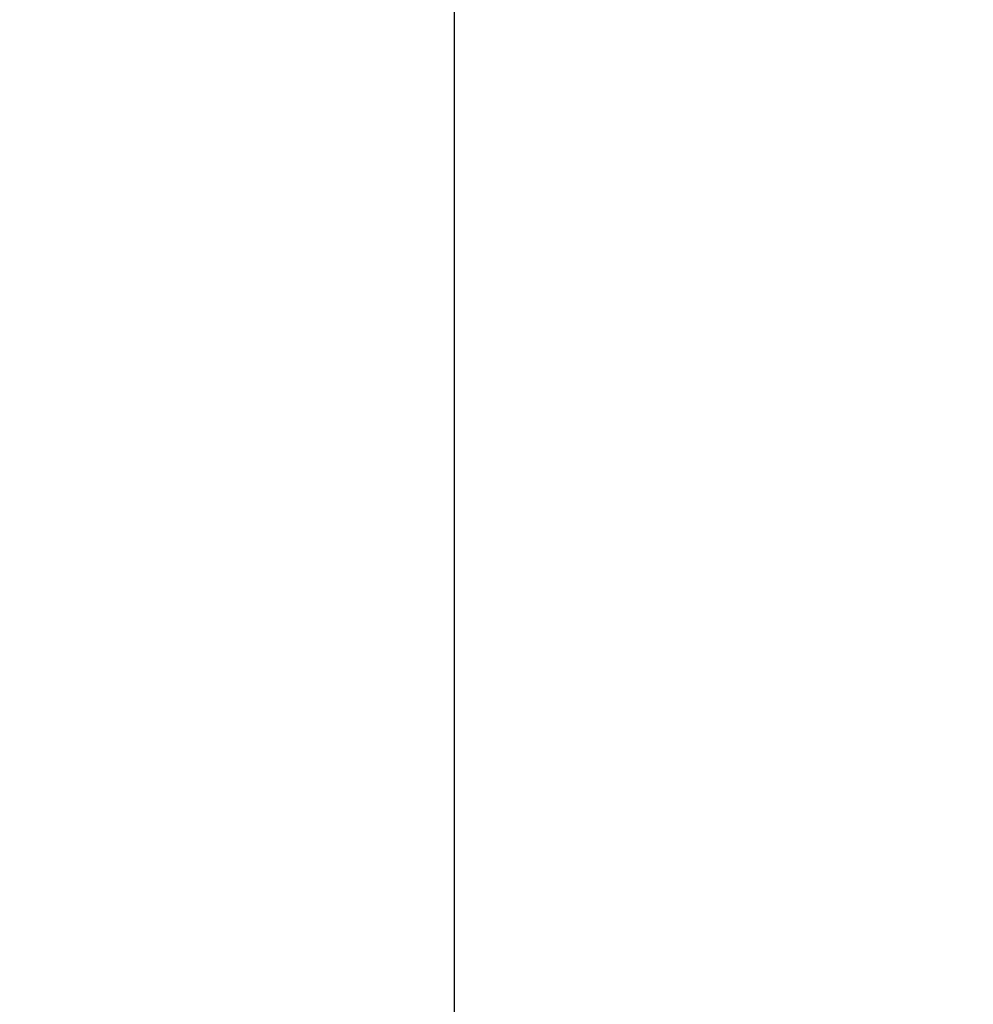
# Model space of a CAD drawing. Units: inches. Extents: x 2083 to 3317, y 1141 to 2115.
# Tile 125 of 256: x 3119.67 to 3135.66, y 1238.34 to 1254.86. Entities that reach past the tile are written whole.
import ezdxf

# ---------------------------------------------------------------- set-up
doc = ezdxf.new("R2010")
doc.units = ezdxf.units.IN
doc.layers.add('A-ANNO-DIMS', color=2, linetype='Continuous', lineweight=18)
doc.styles.get("Standard").update_dxf_attribs({"font": 'arial.ttf'})
doc.dimstyles.new('ISO-25', dxfattribs={"dimtxt": 12, "dimasz": 12, "dimexe": 1.25, "dimexo": 0.625, "dimtad": 1, "dimlunit": 3, "dimtxsty": 'Standard', "dimcen": 2.5, "dimadec": 0, "dimazin": 0, "dimtfac": 1, "dimtmove": 0, "dimatfit": 3, "dimfxl": 1, "dimarcsym": 0})

# ---------------------------------------------------------------- blocks, each defined once
blk = doc.blocks.new('*D10')
at = {"layer": 'A-ANNO-DIMS', "color": 0, "lineweight": -2, "transparency": 16777216}
for p, q in [((2862.96, 1262.636), (2862.96, 1201.384)), ((3126.96, 1262.636), (3126.96, 1201.384)), ((2874.96, 1202.634), (3114.96, 1202.634))]:
    blk.add_line(p, q, dxfattribs=at)
at = {"layer": 'A-ANNO-DIMS', "color": 0, "transparency": 16777216}
for points in [[(2874.96, 1204.634), (2874.96, 1200.634), (2862.96, 1202.634)], [(3114.96, 1204.634), (3114.96, 1200.634), (3126.96, 1202.634)]]:
    blk.add_solid(points, dxfattribs=at)
at = {"layer": 'Defpoints', "color": 0, "transparency": 16777216}
for p in [(2862.96, 1263.261), (3126.96, 1263.261), (3126.96, 1202.634)]:
    blk.add_point(p, dxfattribs=at)
at = {"layer": 'A-ANNO-DIMS', "color": 0, "transparency": 16777216, "insert": (2994.96, 1209.284), "char_height": 12, "attachment_point": 5}
blk.add_mtext("22'", dxfattribs=at)
blk = doc.blocks.new('*D26')
at = {"layer": 'A-ANNO-DIMS', "color": 0, "lineweight": -2, "transparency": 16777216}
for p, q in [((3088.986, 1274.915), (3088.986, 1270.952)), ((3111.24, 1274.915), (3111.24, 1270.952)), ((3076.986, 1272.202), (2840.262, 1272.202)), ((3111.24, 1272.202), (3088.986, 1272.202)), ((3123.24, 1272.202), (3135.24, 1272.202))]:
    blk.add_line(p, q, dxfattribs=at)
at = {"layer": 'A-ANNO-DIMS', "color": 0, "transparency": 16777216}
for points in [[(3076.986, 1274.202), (3076.986, 1270.202), (3088.986, 1272.202)], [(3123.24, 1274.202), (3123.24, 1270.202), (3111.24, 1272.202)]]:
    blk.add_solid(points, dxfattribs=at)
at = {"layer": 'Defpoints', "color": 0, "transparency": 16777216}
for p in [(3088.986, 1275.54), (3111.24, 1275.54), (3088.986, 1272.202)]:
    blk.add_point(p, dxfattribs=at)
at = {"layer": 'A-ANNO-DIMS', "color": 0, "transparency": 16777216, "insert": (2952.624, 1279.032), "char_height": 12, "attachment_point": 5}
blk.add_mtext('NIGHTSTAND 1\'-10 1/2" TYP.', dxfattribs=at)
blk = doc.blocks.new('*D27')
at = {"layer": 'A-ANNO-DIMS', "color": 0, "lineweight": -2, "transparency": 16777216}
for p, q in [((3114.578, 1309.794), (3114.578, 1321.794)), ((3111.865, 1297.794), (3115.828, 1297.794)), ((3114.578, 1297.794), (3114.578, 1275.54)), ((3111.865, 1275.54), (3115.828, 1275.54)), ((3114.578, 1263.54), (3114.578, 1140.989))]:
    blk.add_line(p, q, dxfattribs=at)
at = {"layer": 'A-ANNO-DIMS', "color": 0, "transparency": 16777216}
for points in [[(3112.578, 1309.794), (3116.578, 1309.794), (3114.578, 1297.794)], [(3112.578, 1263.54), (3116.578, 1263.54), (3114.578, 1275.54)]]:
    blk.add_solid(points, dxfattribs=at)
at = {"layer": 'Defpoints', "color": 0, "transparency": 16777216}
for p in [(3111.24, 1297.794), (3111.24, 1275.54), (3114.578, 1275.54)]:
    blk.add_point(p, dxfattribs=at)
at = {"layer": 'A-ANNO-DIMS', "color": 0, "transparency": 16777216, "insert": (3107.749, 1196.264), "char_height": 12, "attachment_point": 5, "rotation": 90}
blk.add_mtext('1\'-10 1/2" TYP.', dxfattribs=at)
blk = doc.blocks.new('*D34')
at = {"layer": 'A-ANNO-DIMS', "color": 0, "lineweight": -2, "transparency": 16777216}
for p, q in [((2226.96, 1262.636), (2226.96, 1209.661)), ((3126.96, 1262.636), (3126.96, 1209.661)), ((2238.96, 1210.911), (3114.96, 1210.911))]:
    blk.add_line(p, q, dxfattribs=at)
at = {"layer": 'A-ANNO-DIMS', "color": 0, "transparency": 16777216}
for points in [[(2238.96, 1212.911), (2238.96, 1208.911), (2226.96, 1210.911)], [(3114.96, 1212.911), (3114.96, 1208.911), (3126.96, 1210.911)]]:
    blk.add_solid(points, dxfattribs=at)
at = {"layer": 'Defpoints', "color": 0, "transparency": 16777216}
for p in [(2226.96, 1263.261), (3126.96, 1263.261), (3126.96, 1210.911)]:
    blk.add_point(p, dxfattribs=at)
at = {"layer": 'A-ANNO-DIMS', "color": 0, "transparency": 16777216, "insert": (2676.96, 1217.663), "char_height": 12, "attachment_point": 5}
blk.add_mtext('75\'-0"', dxfattribs=at)

msp = doc.modelspace()

# ---------------------------------------------------------------- dimensions: what is measured, and where the dimension line sits
at = {"layer": 'A-ANNO-DIMS'}
for base, p1, p2, angle, text, picture, middle in [((3114.578, 1275.54), (3111.24, 1297.794), (3111.24, 1275.54), 270, '<> TYP.', '*D27', (3107.749, 1196.264)), ((3088.986, 1272.202), (3111.24, 1275.54), (3088.986, 1275.54), 180, 'NIGHTSTAND <> TYP.', '*D26', (2952.624, 1279.032))]:
    dim = msp.add_linear_dim(base=base, p1=p1, p2=p2, angle=angle, text=text, dimstyle='ISO-25', override={"dimdec": 1, "dimlfac": 1, "dimrnd": 0, "dimzin": 1, "dimdsep": 46, "dimlunit": 4, "dimfrac": 2}, dxfattribs=at)
    dim.commit()
    dim.dimension.update_dxf_attribs({"geometry": picture, "text_midpoint": middle})
for base, p1, override, picture, middle in [((3126.96, 1210.911), (2226.96, 1263.261), {"dimdec": 1, "dimlfac": 1, "dimrnd": 0, "dimzin": 1, "dimdsep": 46, "dimlunit": 4, "dimfrac": 2}, '*D34', (2676.96, 1217.663)), ((3126.96, 1202.634), (2862.96, 1263.261), {"dimclrd": 0, "dimclre": 0, "dimclrt": 0}, '*D10', (2994.96, 1209.284))]:
    dim = msp.add_linear_dim(base=base, p1=p1, p2=(3126.96, 1263.261), dimstyle='ISO-25', override=override, dxfattribs=at)
    dim.commit()
    dim.dimension.update_dxf_attribs({"geometry": picture, "text_midpoint": middle})

doc.saveas('drawing.dxf')
